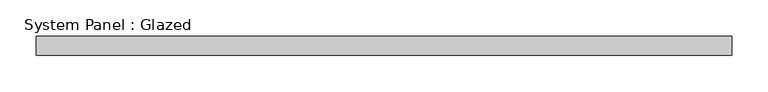
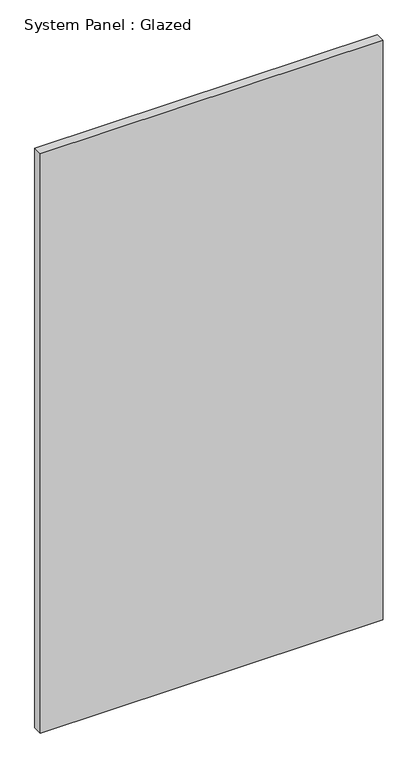
"""IFC4 building model written with IfcOpenShell, lengths in millimetres: plate geometry, System Panel : Glazed."""

from ifc_helpers import new_model, si_unit, origin, origin_with_axes, place, context, project, spatial, polyline, outline, extrude, source, transform, mapped, element, save


def system_panel_glazed_0f092676(model_context):
    return source(origin(), model_context, "Body", "SweptSolid", [
        extrude(outline(polyline([(476.3558776, 19.05), (-476.3558776, 19.05), (-476.3558776, 44.45), (476.3558776, 44.45), (476.3558776, 19.05)])), origin_with_axes(), (0.0, 0.0, 1.0), 1701.8),
    ])


if __name__ == "__main__":
    model = new_model("IFC4")
    model_context = context("Model", 3, world=origin())
    ifc_project = project(units=[si_unit("LENGTHUNIT", "METRE", prefix="MILLI")], contexts=[model_context])
    site = spatial("IfcSite", under=ifc_project)
    building = spatial("IfcBuilding", under=site)
    placement = place(None, origin())
    system_panel_glazed_shape = system_panel_glazed_0f092676(model_context)
    element("IfcPlate", 1, ObjectType="System Panel : Glazed", at=placement, inside=building, context=model_context, shape_type="MappedRepresentation", body=[
        mapped(system_panel_glazed_shape, transform((0.0, 0.0, 0.0), x_axis=(1.0, 0.0, 0.0), y_axis=(0.0, 1.0, 0.0), z_axis=(0.0, 0.0, 1.0))),
    ])
    save(model, "model.ifc")

# Revit data of these elements
# Type "System Panel : Glazed"
#   Construction Type Id = "GSP4R"
#   Analytic Construction = "1/8 in Pilkington single glazing"
#   Visual Light Transmittance = 0.9
#   Solar Heat Gain Coefficient = 0.86
#   Heat Transfer Coefficient (U) = 1.18115 BTU/(h·ft²·°F)
#   Define Thermal Properties by = 1
# Element 1 (IfcPlate, "System Panel : Glazed")
#   Materials on its faces: "Glass"
# Materials
#   "Glass": class "Glass", colour RGB 154 182 205, transparency 0.85, Description = "Soda Lime Glass", Cost = 0
